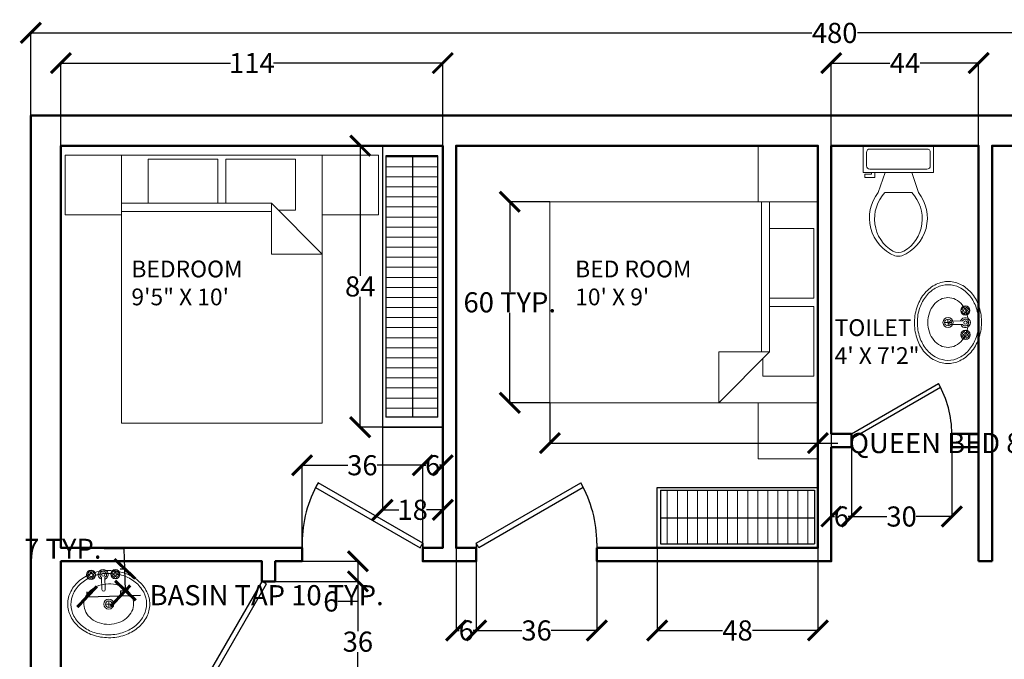
# Model space of a CAD drawing. Units: inches. Extents: x 9 to 573, y -373 to 44.
# Tile 3 of 5: x 35 to 329, y -146 to 44. Entities that reach past the tile are written whole.
import ezdxf

# ---------------------------------------------------------------- set-up
doc = ezdxf.new("R2010")
doc.units = ezdxf.units.IN
doc.header["$MEASUREMENT"] = 0
for name, color, linetype, lineweight in [('A-ANNO-DIMS', 2, 'Continuous', 18), ('A-AREA-IDEN', 7, 'Continuous', 25), ('A-DOOR', 4, 'Continuous', 25), ('A-FLOR-CASE', 8, 'Continuous', 25), ('A-FLOR-CASE-PATT', 252, 'Continuous', 13), ('A-FLOR-FIXT', 9, 'Continuous', 18), ('A-FURN', 8, 'Continuous', 18), ('A-WALL', 7, 'Continuous', 50)]:
    doc.layers.add(name, color=color, linetype=linetype, lineweight=lineweight)
doc.styles.get("Standard").update_dxf_attribs({"font": 'arial.ttf'})
doc.dimstyles.get("Standard").update_dxf_attribs({"dimtxt": 6, "dimasz": 6, "dimexe": 0.18, "dimexo": 0.0625, "dimgap": 0.09, "dimtad": 0, "dimtih": 1, "dimtoh": 1, "dimdec": 0, "dimzin": 0, "dimdsep": 46, "dimlunit": 4, "dimtxsty": 'Standard', "dimblk": 'ARCHTICK', "dimcen": 0.09, "dimadec": 0, "dimazin": 0, "dimtfac": 1, "dimtdec": 0, "dimtofl": 0, "dimtmove": 0, "dimatfit": 3, "dimldrblk": 'ARCHTICK', "dimfxl": 1, "dimtolj": 1, "dimtzin": 0, "dimarcsym": 0})

# ---------------------------------------------------------------- blocks, each defined once
blk = doc.blocks.new('*U5')
for p, q in [((0, 0), (0, -6)), ((-40, 0), (-40, -6))]:
    blk.add_line(p, q)
blk.add_lwpolyline([(0, 0), (-34.64, 20), (-35.52, 18.48), (-0.88, -1.52)], close=True)
blk.add_arc((0, 0), 40, 150, 180)
blk = doc.blocks.new('*U4')
for p, q in [((0, 0), (0, -6)), ((40, 0), (40, -6))]:
    blk.add_line(p, q)
blk.add_lwpolyline([(0, 0), (34.64, 20), (35.52, 18.48), (0.88, -1.52)], close=True)
blk.add_arc((0, 0), 40, 0, 30)
blk = doc.blocks.new('*U7')
for p, q in [((0, 0), (0, -6)), ((40, 0), (40, -6))]:
    blk.add_line(p, q)
blk.add_lwpolyline([(0, 0), (34.64, 20), (35.52, 18.48), (0.87, -1.52)], close=True)
blk.add_arc((0, 0), 40, 0, 30)
blk = doc.blocks.new('Bed - Queen')
for p, q in [((0, -80.00003), (0, 0)), ((0, 0), (59.99999, 0)), ((59.99999, 0), (59.99999, -80.00003)), ((7.99999, -1.2), (28.79998, -1.2)), ((7.99999, -14.4), (7.99999, -1.2)), ((28.79998, -1.2), (28.79998, -14.4)), ((31.19999, -1.2), (51.99999, -1.2)), ((31.19999, -14.4), (31.19999, -1.2)), ((51.99999, -1.2), (51.99999, -16.4)), ((0, -14.4), (44.8, -14.4)), ((59.99999, -29.6), (44.8, -14.4)), ((44.8, -14.4), (44.8, -29.6)), ((44.8, -16.8), (0, -16.8)), ((51.99999, -16.4), (46.79936, -16.4)), ((44.8, -29.6), (59.99999, -29.6)), ((59.99999, -80.00003), (0, -80.00003))]:
    blk.add_line(p, q)
blk = doc.blocks.new('Toilet - top')
for p, q in [((9.5, -6), (9.5, -2)), ((-10, -8.5), (-8, -8.5)), ((-10, -9.5), (-10, -8.5)), ((-8, -8.5), (-8, -8)), ((-7, -8), (-7, -9.5)), ((-4, -8), (-6, -14)), ((4, -8), (6, -14)), ((-7, -9.5), (-10, -9.5)), ((4, -14), (-4, -14))]:
    blk.add_line(p, q)
blk.add_lwpolyline([(10.5, -8), (10.5, 0), (-10.5, 0), (-10.5, -8)], close=True)
for points in [[(-9.5, -2), (-9.5, -6)], [(8.5, -1), (-8.5, -1)], [(-8.5, -7), (8.5, -7)]]:
    blk.add_lwpolyline(points)
for centre, radius, start, end in [((-8.62, -1.88), 0.884, 81.8699, 188.1301), ((8.62, -1.88), 0.884, 351.8699, 98.1301), ((-8.62, -6.12), 0.884, 171.8699, 278.1301), ((8.62, -6.12), 0.884, 261.8699, 8.1301), ((3.52, -21.58), 12.17, 141.4691, 247.9714), ((4.2, -21.82), 11.33, 136.3677, 238.9468), ((-3.52, -21.58), 12.17, 292.0284, 38.5307), ((-4.2, -21.82), 11.33, 301.053, 43.6321), ((0, -27.88), 4, 245.7318, 294.2682), ((0, -29), 4, 254.8605, 285.1395)]:
    blk.add_arc(centre, radius, start, end)
blk = doc.blocks.new('Sink - Oval top')
for p, q in [((-1, 0), (1, 0)), ((0, 1), (0, -1))]:
    blk.add_line(p, q)
for points in [[(-12.23, 0.39, 0.117634), (-11.46, -3.36, 0.104469), (-8.88, -6.8, 0.090016), (-5.08, -9.07, 0.08192), (-0.32, -10.02, 0.08192), (4.49, -9.38, 0.090016), (8.42, -7.36, 0.104469), (11.22, -4.09, 0.117634), (12.23, -0.39, 0.117634), (11.46, 3.36, 0.104469), (8.88, 6.8, 0.090016), (5.08, 9.07, 0.08192), (0.32, 10.02, 0.08192), (-4.49, 9.38, 0.090016), (-8.42, 7.36, 0.104469), (-11.22, 4.09, 0.117634)], [(-11.29, 0.16, 0.118622), (-10.52, -3.25, 0.104678), (-8.07, -6.36, 0.089562), (-4.54, -8.37, 0.081185), (-0.13, -9.15, 0.081185), (4.3, -8.49, 0.089562), (7.89, -6.58, 0.104678), (10.42, -3.55, 0.118622), (11.29, -0.16, 0.118622), (10.52, 3.25, 0.104678), (8.07, 6.36, 0.089562), (4.54, 8.37, 0.081185), (0.13, 9.15, 0.081185), (-4.3, 8.49, 0.089562), (-7.89, 6.58, 0.104678), (-10.42, 3.55, 0.118622)], [(-7.42, 0.08, 0.118283), (-6.91, -2.17, 0.104607), (-5.29, -4.21, 0.089718), (-2.97, -5.53, 0.081436), (-0.07, -6.04, 0.081436), (2.84, -5.59, 0.089718), (5.2, -4.33, 0.104607), (6.86, -2.32, 0.118283), (7.42, -0.08, 0.118283), (6.91, 2.17, 0.104607), (5.29, 4.21, 0.089718), (2.97, 5.53, 0.081436), (0.07, 6.04, 0.081436), (-2.84, 5.59, 0.089718), (-5.2, 4.33, 0.104607), (-6.86, 2.32, 0.118283)]]:
    blk.add_lwpolyline(points, format="xyb", close=True)
for radius in [1.5, 1]:
    blk.add_circle((0, 0), radius)
blk = doc.blocks.new('Faucet - Bathroom top')
for p, q in [((-4.107, 0.125), (-4.375, 0.125)), ((-3.75, 0.4788), (-3.75, 0.75)), ((-3.5, 0.482), (-3.5, 0.75)), ((-3.1461, 0.125), (-2.875, 0.125)), ((3.143, 0.125), (2.875, 0.125)), ((3.5, 0.4788), (3.5, 0.75)), ((3.75, 0.482), (3.75, 0.75)), ((4.1039, 0.125), (4.375, 0.125)), ((-4.1039, -0.125), (-4.375, -0.125)), ((-3.75, -0.4821), (-3.75, -0.75)), ((-3.5, -0.4789), (-3.5, -0.75)), ((-3.143, -0.125), (-2.875, -0.125)), ((-0.5, -0.8639), (-0.5, -4.5)), ((0.5, -4.5), (0.5, -0.8631)), ((3.1461, -0.125), (2.875, -0.125)), ((3.5, -0.4821), (3.5, -0.75)), ((3.75, -0.4789), (3.75, -0.75)), ((4.107, -0.125), (4.375, -0.125))]:
    blk.add_line(p, q)
for centre, radius in [((-3.625, 0), 1.375), ((-4.625, 0), 0.2795), ((-3.625, 0), 0.5), ((-3.625, 1), 0.2795), ((-2.625, 0), 0.2795), ((0, 0), 0.5), ((3.625, 0), 1.375), ((2.625, 0), 0.2795), ((3.625, 0), 0.5), ((3.625, 1), 0.2795), ((4.625, 0), 0.2795), ((-3.625, -1), 0.2795), ((3.625, -1), 0.2795)]:
    blk.add_circle(centre, radius)
for centre, radius, start, end in [((-3.625, 0), 1, 105.2407, 164.2093), ((-3.625, 0), 1, 16.44125, 74.07887), ((0, 0), 1.5, 289.6514, 250.3603), ((0, 0), 1, 300.3431, 239.7554), ((3.625, 0), 1, 106.12, 164.0884), ((3.625, 0), 1, 16.23422, 73.90469), ((-3.625, 0), 1, 196.2342, 253.9047), ((-3.625, 0), 1, 286.12, 344.0884), ((3.625, 0), 1, 196.4413, 254.0789), ((3.625, 0), 1, 285.2407, 344.2093), ((0, -4.5), 0.5, 180, 0)]:
    blk.add_arc(centre, radius, start, end)
blk = doc.blocks.new('*U25')
for p, q in [((0, 0), (0, 6)), ((40, 0), (40, 6))]:
    blk.add_line(p, q)
blk.add_lwpolyline([(0, 0), (34.64, -20), (35.52, -18.48), (0.87, 1.52)], close=True)
blk.add_arc((0, 0), 40, 330, 0)
blk = doc.blocks.new('BEDSIDE-TABLE')
blk.add_lwpolyline([(0, 17.82), (16.74, 17.82), (16.74, 0), (0, 0)], close=True)
blk = doc.blocks.new('_ArchTick')
at = {"color": 0, "linetype": 'ByBlock', "const_width": 0.15}
blk.add_lwpolyline([(-0.5, -0.5), (0.5, 0.5)], dxfattribs=at)
blk = doc.blocks.new('*D30')
at = {"layer": 'A-ANNO-DIMS', "color": 0, "lineweight": -2, "transparency": 16777216}
for p, q in [((193.52, -70), (193.52, -82.12)), ((273.52, -70), (273.52, -82.12)), ((193.52, -81.94), (273.52, -81.94)), ((273.52, -81.94), (279.52, -81.94))]:
    blk.add_line(p, q, dxfattribs=at)
at = {"layer": 'Defpoints', "color": 0, "transparency": 16777216}
for p in [(193.52, -69.94), (273.52, -69.94), (273.52, -81.94)]:
    blk.add_point(p, dxfattribs=at)
at = {"layer": 'A-ANNO-DIMS', "color": 0, "lineweight": -2, "transparency": 16777216, "xscale": 6, "yscale": 6, "zscale": 6, "rotation": 180}
blk.add_blockref('_ArchTick', (193.52, -81.94), dxfattribs=at)
at = {"layer": 'A-ANNO-DIMS', "color": 0, "lineweight": -2, "transparency": 16777216, "xscale": 6, "yscale": 6, "zscale": 6}
blk.add_blockref('_ArchTick', (273.52, -81.94), dxfattribs=at)
at = {"layer": 'A-ANNO-DIMS', "color": 0, "transparency": 16777216, "insert": (320.05, -81.94), "char_height": 6, "attachment_point": 5}
blk.add_mtext('\\A1;QUEEN BED 80 TYP.', dxfattribs=at)
blk = doc.blocks.new('*D31')
at = {"layer": 'A-ANNO-DIMS', "color": 0, "lineweight": -2, "transparency": 16777216}
for p, q in [((193.45, -9.94), (181.34, -9.94)), ((181.52, -9.94), (181.52, -36.78)), ((181.52, -69.94), (181.52, -43.09)), ((193.45, -69.94), (181.34, -69.94))]:
    blk.add_line(p, q, dxfattribs=at)
at = {"layer": 'Defpoints', "color": 0, "transparency": 16777216}
for p in [(193.52, -9.94), (181.52, -69.94), (193.52, -69.94)]:
    blk.add_point(p, dxfattribs=at)
at = {"layer": 'A-ANNO-DIMS', "color": 0, "lineweight": -2, "transparency": 16777216, "xscale": 6, "yscale": 6, "zscale": 6}
for p, rotation in [((181.52, -9.94), 90), ((181.52, -69.94), 270)]:
    blk.add_blockref('_ArchTick', p, dxfattribs=dict(at, rotation=rotation))
at = {"layer": 'A-ANNO-DIMS', "color": 0, "transparency": 16777216, "insert": (181.52, -39.94), "char_height": 6, "attachment_point": 5}
blk.add_mtext('\\A1;60 TYP.', dxfattribs=at)
blk = doc.blocks.new('*D40')
at = {"layer": 'A-ANNO-DIMS', "color": 0, "lineweight": -2, "transparency": 16777216}
for p, q in [((55.28, -126.35), (55.32, -127.97)), ((65.27, -126.07), (65.32, -127.68)), ((55.32, -127.79), (65.31, -127.5)), ((65.31, -127.5), (71.31, -127.33))]:
    blk.add_line(p, q, dxfattribs=at)
at = {"layer": 'Defpoints', "color": 0, "transparency": 16777216}
for p in [(55.28, -126.29), (65.27, -126.01), (65.31, -127.5)]:
    blk.add_point(p, dxfattribs=at)
at = {"layer": 'A-ANNO-DIMS', "color": 0, "lineweight": -2, "transparency": 16777216, "xscale": 6, "yscale": 6, "zscale": 6}
for p, rotation in [((55.32, -127.79), 181.633858055105), ((65.31, -127.5), 1.633858055105019)]:
    blk.add_blockref('_ArchTick', p, dxfattribs=dict(at, rotation=rotation))
at = {"layer": 'A-ANNO-DIMS', "color": 0, "transparency": 16777216, "insert": (108.93, -127.33), "char_height": 6, "attachment_point": 5}
blk.add_mtext('\\A1;BASIN TAP 10 TYP.', dxfattribs=at)
blk = doc.blocks.new('*D41')
at = {"layer": 'A-ANNO-DIMS', "color": 0, "lineweight": -2, "transparency": 16777216}
for p, q in [((66.41, -113.47), (60.41, -113.47)), ((66.59, -119.47), (66.41, -113.47)), ((65.15, -119.51), (66.77, -119.46)), ((66.77, -125.96), (66.59, -119.47)), ((65.33, -126), (66.95, -125.96))]:
    blk.add_line(p, q, dxfattribs=at)
at = {"layer": 'Defpoints', "color": 0, "transparency": 16777216}
for p in [(65.09, -119.51), (66.59, -119.47), (65.27, -126.01)]:
    blk.add_point(p, dxfattribs=at)
at = {"layer": 'A-ANNO-DIMS', "color": 0, "lineweight": -2, "transparency": 16777216, "xscale": 6, "yscale": 6, "zscale": 6}
for p, rotation in [((66.59, -119.47), 91.63385805510502), ((66.77, -125.96), 271.633858055105)]:
    blk.add_blockref('_ArchTick', p, dxfattribs=dict(at, rotation=rotation))
at = {"layer": 'A-ANNO-DIMS', "color": 0, "transparency": 16777216, "insert": (48.08, -113.47), "char_height": 6, "attachment_point": 5}
blk.add_mtext('\\A1;7 TYP.', dxfattribs=at)
blk = doc.blocks.new('*D58')
at = {"layer": 'A-ANNO-DIMS', "color": 0, "lineweight": -2, "transparency": 16777216}
for p, q in [((38.52, 15.87), (38.52, 40.63)), ((38.52, 40.45), (271.69, 40.45)), ((518.52, 40.45), (285.35, 40.45)), ((518.52, 15.87), (518.52, 40.63))]:
    blk.add_line(p, q, dxfattribs=at)
at = {"layer": 'Defpoints', "color": 0, "transparency": 16777216}
for p in [(518.52, 40.45), (38.52, 15.8), (518.52, 15.8)]:
    blk.add_point(p, dxfattribs=at)
at = {"layer": 'A-ANNO-DIMS', "color": 0, "lineweight": -2, "transparency": 16777216, "xscale": 6, "yscale": 6, "zscale": 6, "rotation": 180}
blk.add_blockref('_ArchTick', (38.52, 40.45), dxfattribs=at)
at = {"layer": 'A-ANNO-DIMS', "color": 0, "lineweight": -2, "transparency": 16777216, "xscale": 6, "yscale": 6, "zscale": 6}
blk.add_blockref('_ArchTick', (518.52, 40.45), dxfattribs=at)
at = {"layer": 'A-ANNO-DIMS', "color": 0, "transparency": 16777216, "insert": (278.52, 40.45), "char_height": 6, "attachment_point": 5}
blk.add_mtext('\\A1;480', dxfattribs=at)
blk = doc.blocks.new('*D68')
at = {"layer": 'A-ANNO-DIMS', "color": 0, "lineweight": -2, "transparency": 16777216}
for p, q in [((277.52, 6.87), (277.52, 31.63)), ((277.52, 31.45), (295.02, 31.45)), ((321.52, 31.45), (304.01, 31.45)), ((321.52, 6.87), (321.52, 31.63))]:
    blk.add_line(p, q, dxfattribs=at)
at = {"layer": 'Defpoints', "color": 0, "transparency": 16777216}
for p in [(321.52, 31.45), (277.52, 6.8), (321.52, 6.8)]:
    blk.add_point(p, dxfattribs=at)
at = {"layer": 'A-ANNO-DIMS', "color": 0, "lineweight": -2, "transparency": 16777216, "xscale": 6, "yscale": 6, "zscale": 6, "rotation": 180}
blk.add_blockref('_ArchTick', (277.52, 31.45), dxfattribs=at)
at = {"layer": 'A-ANNO-DIMS', "color": 0, "lineweight": -2, "transparency": 16777216, "xscale": 6, "yscale": 6, "zscale": 6}
blk.add_blockref('_ArchTick', (321.52, 31.45), dxfattribs=at)
at = {"layer": 'A-ANNO-DIMS', "color": 0, "transparency": 16777216, "insert": (299.52, 31.45), "char_height": 6, "attachment_point": 5}
blk.add_mtext('\\A1;44', dxfattribs=at)
blk = doc.blocks.new('*D69')
at = {"layer": 'A-ANNO-DIMS', "color": 0, "lineweight": -2, "transparency": 16777216}
for p, q in [((47.52, 6.87), (47.52, 31.63)), ((47.52, 31.45), (98.09, 31.45)), ((161.52, 31.45), (110.94, 31.45)), ((161.52, 6.87), (161.52, 31.63))]:
    blk.add_line(p, q, dxfattribs=at)
at = {"layer": 'Defpoints', "color": 0, "transparency": 16777216}
for p in [(161.52, 31.45), (47.52, 6.8), (161.52, 6.8)]:
    blk.add_point(p, dxfattribs=at)
at = {"layer": 'A-ANNO-DIMS', "color": 0, "lineweight": -2, "transparency": 16777216, "xscale": 6, "yscale": 6, "zscale": 6, "rotation": 180}
blk.add_blockref('_ArchTick', (47.52, 31.45), dxfattribs=at)
at = {"layer": 'A-ANNO-DIMS', "color": 0, "lineweight": -2, "transparency": 16777216, "xscale": 6, "yscale": 6, "zscale": 6}
blk.add_blockref('_ArchTick', (161.52, 31.45), dxfattribs=at)
at = {"layer": 'A-ANNO-DIMS', "color": 0, "transparency": 16777216, "insert": (104.52, 31.45), "char_height": 6, "attachment_point": 5}
blk.add_mtext('\\A1;114', dxfattribs=at)
blk = doc.blocks.new('*D70')
at = {"layer": 'A-ANNO-DIMS', "color": 0, "lineweight": -2, "transparency": 16777216}
for p, q in [((119.52, -113.13), (119.52, -88.37)), ((119.52, -88.55), (133.13, -88.55)), ((155.52, -88.55), (141.9, -88.55)), ((155.52, -113.13), (155.52, -88.37))]:
    blk.add_line(p, q, dxfattribs=at)
at = {"layer": 'Defpoints', "color": 0, "transparency": 16777216}
for p in [(155.52, -88.55), (119.52, -113.2), (155.52, -113.2)]:
    blk.add_point(p, dxfattribs=at)
at = {"layer": 'A-ANNO-DIMS', "color": 0, "lineweight": -2, "transparency": 16777216, "xscale": 6, "yscale": 6, "zscale": 6, "rotation": 180}
blk.add_blockref('_ArchTick', (119.52, -88.55), dxfattribs=at)
at = {"layer": 'A-ANNO-DIMS', "color": 0, "lineweight": -2, "transparency": 16777216, "xscale": 6, "yscale": 6, "zscale": 6}
blk.add_blockref('_ArchTick', (155.52, -88.55), dxfattribs=at)
at = {"layer": 'A-ANNO-DIMS', "color": 0, "transparency": 16777216, "insert": (137.52, -88.55), "char_height": 6, "attachment_point": 5}
blk.add_mtext('\\A1;36', dxfattribs=at)
blk = doc.blocks.new('*D71')
at = {"layer": 'A-ANNO-DIMS', "color": 0, "lineweight": -2, "transparency": 16777216}
for p, q in [((155.52, -113.13), (155.52, -88.37)), ((155.52, -88.55), (156.45, -88.55)), ((161.52, -88.55), (160.59, -88.55)), ((161.52, -113.13), (161.52, -88.37))]:
    blk.add_line(p, q, dxfattribs=at)
at = {"layer": 'Defpoints', "color": 0, "transparency": 16777216}
for p in [(161.52, -88.55), (155.52, -113.2), (161.52, -113.2)]:
    blk.add_point(p, dxfattribs=at)
at = {"layer": 'A-ANNO-DIMS', "color": 0, "lineweight": -2, "transparency": 16777216, "xscale": 6, "yscale": 6, "zscale": 6, "rotation": 180}
blk.add_blockref('_ArchTick', (155.52, -88.55), dxfattribs=at)
at = {"layer": 'A-ANNO-DIMS', "color": 0, "lineweight": -2, "transparency": 16777216, "xscale": 6, "yscale": 6, "zscale": 6}
blk.add_blockref('_ArchTick', (161.52, -88.55), dxfattribs=at)
at = {"layer": 'A-ANNO-DIMS', "color": 0, "transparency": 16777216, "insert": (158.52, -88.55), "char_height": 6, "attachment_point": 5}
blk.add_mtext('\\A1;6', dxfattribs=at)
blk = doc.blocks.new('*D72')
at = {"layer": 'A-ANNO-DIMS', "color": 0, "lineweight": -2, "transparency": 16777216}
for p, q in [((283.52, -79.26), (283.52, -104.03)), ((313.52, -79.26), (313.52, -104.03)), ((283.52, -103.85), (294.14, -103.85)), ((313.52, -103.85), (302.89, -103.85))]:
    blk.add_line(p, q, dxfattribs=at)
at = {"layer": 'Defpoints', "color": 0, "transparency": 16777216}
for p in [(283.52, -79.2), (313.52, -79.2), (283.52, -103.85)]:
    blk.add_point(p, dxfattribs=at)
at = {"layer": 'A-ANNO-DIMS', "color": 0, "lineweight": -2, "transparency": 16777216, "xscale": 6, "yscale": 6, "zscale": 6, "rotation": 180}
blk.add_blockref('_ArchTick', (283.52, -103.85), dxfattribs=at)
at = {"layer": 'A-ANNO-DIMS', "color": 0, "lineweight": -2, "transparency": 16777216, "xscale": 6, "yscale": 6, "zscale": 6}
blk.add_blockref('_ArchTick', (313.52, -103.85), dxfattribs=at)
at = {"layer": 'A-ANNO-DIMS', "color": 0, "transparency": 16777216, "insert": (298.52, -103.85), "char_height": 6, "attachment_point": 5}
blk.add_mtext('\\A1;30', dxfattribs=at)
blk = doc.blocks.new('*D73')
at = {"layer": 'A-ANNO-DIMS', "color": 0, "lineweight": -2, "transparency": 16777216}
for p, q in [((277.52, -79.26), (277.52, -104.03)), ((283.52, -79.26), (283.52, -104.03)), ((277.52, -103.85), (278.45, -103.85)), ((283.52, -103.85), (282.59, -103.85))]:
    blk.add_line(p, q, dxfattribs=at)
at = {"layer": 'Defpoints', "color": 0, "transparency": 16777216}
for p in [(277.52, -79.2), (283.52, -79.2), (277.52, -103.85)]:
    blk.add_point(p, dxfattribs=at)
at = {"layer": 'A-ANNO-DIMS', "color": 0, "lineweight": -2, "transparency": 16777216, "xscale": 6, "yscale": 6, "zscale": 6}
for p, rotation in [((277.52, -103.85), 179.9999999999999), ((283.52, -103.85), 359.9999999999999)]:
    blk.add_blockref('_ArchTick', p, dxfattribs=dict(at, rotation=rotation))
at = {"layer": 'A-ANNO-DIMS', "color": 0, "transparency": 16777216, "insert": (280.52, -103.85), "char_height": 6, "attachment_point": 5}
blk.add_mtext('\\A1;6', dxfattribs=at)
blk = doc.blocks.new('*D80')
at = {"layer": 'A-ANNO-DIMS', "color": 0, "lineweight": -2, "transparency": 16777216}
for p, q in [((111.58, -123.2), (136.35, -123.2)), ((136.17, -123.2), (136.17, -138.04)), ((136.17, -159.2), (136.17, -144.35)), ((111.58, -159.2), (136.35, -159.2))]:
    blk.add_line(p, q, dxfattribs=at)
at = {"layer": 'Defpoints', "color": 0, "transparency": 16777216}
for p in [(111.52, -123.2), (111.52, -159.2), (136.17, -159.2)]:
    blk.add_point(p, dxfattribs=at)
at = {"layer": 'A-ANNO-DIMS', "color": 0, "lineweight": -2, "transparency": 16777216, "xscale": 6, "yscale": 6, "zscale": 6}
for p, rotation in [((136.17, -123.2), 90), ((136.17, -159.2), 270)]:
    blk.add_blockref('_ArchTick', p, dxfattribs=dict(at, rotation=rotation))
at = {"layer": 'A-ANNO-DIMS', "color": 0, "transparency": 16777216, "insert": (136.17, -141.2), "char_height": 6, "attachment_point": 5}
blk.add_mtext('\\A1;36', dxfattribs=at)
blk = doc.blocks.new('*D81')
at = {"layer": 'A-ANNO-DIMS', "color": 0, "lineweight": -2, "transparency": 16777216}
for p, q in [((111.58, -117.2), (136.35, -117.2)), ((136.17, -117.2), (136.17, -123.2)), ((111.58, -123.2), (136.35, -123.2)), ((136.17, -123.2), (136.17, -129.2)), ((136.17, -129.2), (130.17, -129.2))]:
    blk.add_line(p, q, dxfattribs=at)
at = {"layer": 'Defpoints', "color": 0, "transparency": 16777216}
for p in [(111.52, -117.2), (111.52, -123.2), (136.17, -123.2)]:
    blk.add_point(p, dxfattribs=at)
at = {"layer": 'A-ANNO-DIMS', "color": 0, "lineweight": -2, "transparency": 16777216, "xscale": 6, "yscale": 6, "zscale": 6}
for p, rotation in [((136.17, -117.2), 90), ((136.17, -123.2), 270)]:
    blk.add_blockref('_ArchTick', p, dxfattribs=dict(at, rotation=rotation))
at = {"layer": 'A-ANNO-DIMS', "color": 0, "transparency": 16777216, "insert": (128.1, -129.2), "char_height": 6, "attachment_point": 5}
blk.add_mtext('\\A1;6', dxfattribs=at)
blk = doc.blocks.new('*D82')
at = {"layer": 'A-ANNO-DIMS', "color": 0, "lineweight": -2, "transparency": 16777216}
for p, q in [((165.52, -113.26), (165.52, -138.03)), ((171.52, -113.26), (171.52, -138.03)), ((165.52, -137.85), (166.45, -137.85)), ((171.52, -137.85), (170.59, -137.85))]:
    blk.add_line(p, q, dxfattribs=at)
at = {"layer": 'Defpoints', "color": 0, "transparency": 16777216}
for p in [(165.52, -113.2), (171.52, -113.2), (165.52, -137.85)]:
    blk.add_point(p, dxfattribs=at)
at = {"layer": 'A-ANNO-DIMS', "color": 0, "lineweight": -2, "transparency": 16777216, "xscale": 6, "yscale": 6, "zscale": 6, "rotation": 180}
blk.add_blockref('_ArchTick', (165.52, -137.85), dxfattribs=at)
at = {"layer": 'A-ANNO-DIMS', "color": 0, "lineweight": -2, "transparency": 16777216, "xscale": 6, "yscale": 6, "zscale": 6}
blk.add_blockref('_ArchTick', (171.52, -137.85), dxfattribs=at)
at = {"layer": 'A-ANNO-DIMS', "color": 0, "transparency": 16777216, "insert": (168.52, -137.85), "char_height": 6, "attachment_point": 5}
blk.add_mtext('\\A1;6', dxfattribs=at)
blk = doc.blocks.new('*D83')
at = {"layer": 'A-ANNO-DIMS', "color": 0, "lineweight": -2, "transparency": 16777216}
for p, q in [((171.52, -113.26), (171.52, -138.03)), ((207.52, -113.26), (207.52, -138.03)), ((171.52, -137.85), (185.13, -137.85)), ((207.52, -137.85), (193.9, -137.85))]:
    blk.add_line(p, q, dxfattribs=at)
at = {"layer": 'Defpoints', "color": 0, "transparency": 16777216}
for p in [(171.52, -113.2), (207.52, -113.2), (171.52, -137.85)]:
    blk.add_point(p, dxfattribs=at)
at = {"layer": 'A-ANNO-DIMS', "color": 0, "lineweight": -2, "transparency": 16777216, "xscale": 6, "yscale": 6, "zscale": 6, "rotation": 180}
blk.add_blockref('_ArchTick', (171.52, -137.85), dxfattribs=at)
at = {"layer": 'A-ANNO-DIMS', "color": 0, "lineweight": -2, "transparency": 16777216, "xscale": 6, "yscale": 6, "zscale": 6}
blk.add_blockref('_ArchTick', (207.52, -137.85), dxfattribs=at)
at = {"layer": 'A-ANNO-DIMS', "color": 0, "transparency": 16777216, "insert": (189.52, -137.85), "char_height": 6, "attachment_point": 5}
blk.add_mtext('\\A1;36', dxfattribs=at)
blk = doc.blocks.new('*D88')
at = {"layer": 'A-ANNO-DIMS', "color": 0, "lineweight": -2, "transparency": 16777216}
for p, q in [((161.45, 6.8), (136.69, 6.8)), ((136.87, 6.8), (136.87, -32.04)), ((136.87, -77.2), (136.87, -38.35)), ((161.45, -77.2), (136.69, -77.2))]:
    blk.add_line(p, q, dxfattribs=at)
at = {"layer": 'Defpoints', "color": 0, "transparency": 16777216}
for p in [(136.87, 6.8), (161.52, 6.8), (161.52, -77.2)]:
    blk.add_point(p, dxfattribs=at)
at = {"layer": 'A-ANNO-DIMS', "color": 0, "lineweight": -2, "transparency": 16777216, "xscale": 6, "yscale": 6, "zscale": 6}
for p, rotation in [((136.87, 6.8), 90), ((136.87, -77.2), 270)]:
    blk.add_blockref('_ArchTick', p, dxfattribs=dict(at, rotation=rotation))
at = {"layer": 'A-ANNO-DIMS', "color": 0, "transparency": 16777216, "insert": (136.87, -35.2), "char_height": 6, "attachment_point": 5}
blk.add_mtext('\\A1;84', dxfattribs=at)
blk = doc.blocks.new('*D89')
at = {"layer": 'A-ANNO-DIMS', "color": 0, "lineweight": -2, "transparency": 16777216}
for p, q in [((143.52, -77.26), (143.52, -102.03)), ((161.52, -77.26), (161.52, -102.03)), ((143.52, -101.85), (148.41, -101.85)), ((161.52, -101.85), (156.63, -101.85))]:
    blk.add_line(p, q, dxfattribs=at)
at = {"layer": 'Defpoints', "color": 0, "transparency": 16777216}
for p in [(143.52, -77.2), (161.52, -77.2), (143.52, -101.85)]:
    blk.add_point(p, dxfattribs=at)
at = {"layer": 'A-ANNO-DIMS', "color": 0, "lineweight": -2, "transparency": 16777216, "xscale": 6, "yscale": 6, "zscale": 6, "rotation": 180}
blk.add_blockref('_ArchTick', (143.52, -101.85), dxfattribs=at)
at = {"layer": 'A-ANNO-DIMS', "color": 0, "lineweight": -2, "transparency": 16777216, "xscale": 6, "yscale": 6, "zscale": 6}
blk.add_blockref('_ArchTick', (161.52, -101.85), dxfattribs=at)
at = {"layer": 'A-ANNO-DIMS', "color": 0, "transparency": 16777216, "insert": (152.52, -101.85), "char_height": 6, "attachment_point": 5}
blk.add_mtext('\\A1;18', dxfattribs=at)
blk = doc.blocks.new('*D90')
at = {"layer": 'A-ANNO-DIMS', "color": 0, "lineweight": -2, "transparency": 16777216}
for p, q in [((225.52, -113.26), (225.52, -138.03)), ((273.52, -113.26), (273.52, -138.03)), ((225.52, -137.85), (245, -137.85)), ((273.52, -137.85), (254.03, -137.85))]:
    blk.add_line(p, q, dxfattribs=at)
at = {"layer": 'Defpoints', "color": 0, "transparency": 16777216}
for p in [(225.52, -113.2), (273.52, -113.2), (225.52, -137.85)]:
    blk.add_point(p, dxfattribs=at)
at = {"layer": 'A-ANNO-DIMS', "color": 0, "lineweight": -2, "transparency": 16777216, "xscale": 6, "yscale": 6, "zscale": 6, "rotation": 180}
blk.add_blockref('_ArchTick', (225.52, -137.85), dxfattribs=at)
at = {"layer": 'A-ANNO-DIMS', "color": 0, "lineweight": -2, "transparency": 16777216, "xscale": 6, "yscale": 6, "zscale": 6}
blk.add_blockref('_ArchTick', (273.52, -137.85), dxfattribs=at)
at = {"layer": 'A-ANNO-DIMS', "color": 0, "transparency": 16777216, "insert": (249.52, -137.85), "char_height": 6, "attachment_point": 5}
blk.add_mtext('\\A1;48', dxfattribs=at)

msp = doc.modelspace()

# ---------------------------------------------------------------- hatches: boundary and pattern name
at = {"layer": 'A-FLOR-CASE-PATT'}
h = msp.add_hatch(dxfattribs=at)
h.set_pattern_fill('ANSI31', color=256, scale=24, angle=-45, style=0)
h.set_pattern_definition([(0, (-716.4455, -458.4915), (0, 3), [])])
h.paths.add_polyline_path([(144.5545, -74.1966), (160.0545, -74.1966), (160.0545, 3.8034), (144.5545, 3.8034)])
h = msp.add_hatch(dxfattribs=at)
h.set_pattern_fill('ANSI31', color=256, scale=24, angle=45, style=0)
h.set_pattern_definition([(90, (-716.4455, -458.4915), (-3, 0), [])])
h.paths.add_polyline_path([(226.5545, -111.9915), (272.5545, -111.9915), (272.5545, -95.9915), (226.5545, -95.9915)])

# ---------------------------------------------------------------- linework, layer by layer
at = {"layer": 'A-FLOR-CASE'}
for p, q in [((161.5169, 6.8034), (143.5169, 6.8034)), ((143.5169, 6.8034), (143.5169, -77.1966)), ((161.5169, -77.1966), (161.5169, 6.8034)), ((160.0545, 3.8034), (144.5545, 3.8034)), ((144.5545, 3.8034), (144.5545, -74.1966)), ((152.5169, 3.8034), (152.5169, -74.1966)), ((160.0545, -74.1966), (160.0545, 3.8034)), ((160.0545, -74.1966), (144.5545, -74.1966)), ((143.5169, -77.1966), (161.5169, -77.1966)), ((225.5169, -113.1966), (225.5169, -95.1966)), ((225.5169, -95.1966), (273.5169, -95.1966)), ((226.5545, -95.9915), (272.5545, -95.9915)), ((226.5545, -95.9915), (226.5545, -111.9915)), ((272.5545, -95.9915), (272.5545, -111.9915)), ((273.5169, -95.1966), (273.5169, -113.1966)), ((226.5545, -104.1966), (272.5545, -104.1966)), ((273.5169, -113.1966), (225.5169, -113.1966)), ((226.5545, -111.9915), (272.5545, -111.9915))]:
    msp.add_line(p, q, dxfattribs=at)
at = {"layer": 'A-WALL'}
for p, q in [((283.5169, -79.1966), (283.5169, -83.1966)), ((313.5169, -79.1966), (313.5169, -83.1966)), ((313.5169, -79.1966), (321.5169, -79.1966)), ((313.5169, -83.1966), (321.5169, -83.1966)), ((325.5169, -113.1966), (325.5169, -117.1966))]:
    msp.add_line(p, q, dxfattribs=at)
for points in [[(329.5169, -215.1966), (329.5169, -335.1966), (509.5169, -335.1966), (518.5169, -335.1966), (518.5169, -344.1966), (38.5169, -344.1966), (38.5169, 15.8034), (518.5169, 15.8034), (518.5169, -117.1966), (450.7536, -117.1966), (450.7536, -140.1966), (446.7536, -140.1966), (446.7536, -117.1966), (431.5169, -117.1966), (431.5169, -113.1966), (509.5169, -113.1966), (509.5169, 6.8034), (389.5169, 6.8034), (389.5169, -113.1966), (395.5169, -113.1966), (395.5169, -117.1966), (385.5169, -117.1966), (385.5169, 6.8034), (325.5169, 6.8034)], [(283.5169, -83.1966), (277.5169, -83.1966), (277.5169, -117.1966), (207.5169, -117.1966), (207.5169, -113.1966), (273.5169, -113.1966), (273.5169, 6.8034), (165.5169, 6.8034), (165.5169, -113.1966), (171.5169, -113.1966), (171.5169, -117.1966), (155.5169, -117.1966), (155.5169, -113.1966), (161.5169, -113.1966), (161.5169, 6.8034), (47.5169, 6.8034), (47.5169, -113.1966), (119.5169, -113.1966), (119.5169, -117.1966), (111.5169, -117.1966), (111.5169, -123.1966), (107.5169, -123.1966), (107.5169, -117.1966), (47.5169, -117.1966), (47.5169, -211.1966)], [(321.5169, -117.1966), (321.5169, 6.8034), (277.5169, 6.8034), (277.5169, -79.1966), (283.5169, -79.1966)], [(325.5169, -117.1966), (321.5169, -117.1966)]]:
    msp.add_lwpolyline(points, dxfattribs=at)
msp.add_lwpolyline([(325.5169, -113.1966), (325.5169, 6.8034)], close=True, dxfattribs=at)

# ---------------------------------------------------------------- block references
at = {"layer": 'A-DOOR'}
for name, p, xscale, yscale, zscale in [('*U7', (283.5169, -79.1966), 0.75, 0.75, 0.75), ('*U5', (155.5169, -111.7966), 0.9, 0.9, 0.9), ('*U4', (171.5169, -111.7966), 0.9, 0.9, 0.9)]:
    msp.add_blockref(name, p, dxfattribs=dict(at, xscale=xscale, yscale=yscale, zscale=zscale))
at = {"layer": 'A-DOOR', "xscale": 0.9, "yscale": 0.9, "zscale": 0.9, "rotation": 270}
msp.add_blockref('*U25', (107.5169, -123.1966), dxfattribs=at)
at = {"layer": 'A-FLOR-FIXT'}
msp.add_blockref('Toilet - top', (297.5545, 6.8034), dxfattribs=at)
for name, p, rotation in [('Sink - Oval top', (312.3645, -45.9644), 270.6375101586001), ('Faucet - Bathroom top', (317.5627, -45.9994), 270.6375101586001), ('Sink - Oval top', (61.7933, -129.9889), 1.633858055105068), ('Faucet - Bathroom top', (60.1311, -121.15), 1.633858055105068)]:
    msp.add_blockref(name, p, dxfattribs=dict(at, rotation=rotation))
at = {"layer": 'A-FURN', "rotation": 270}
for name, p in [('BEDSIDE-TABLE', (255.6923, 6.8038)), ('Bed - Queen', (273.5169, -9.9382)), ('BEDSIDE-TABLE', (255.6923, -69.9377))]:
    msp.add_blockref(name, p, dxfattribs=at)
at = {"layer": 'A-FURN'}
for name, p in [('BEDSIDE-TABLE', (48.8124, -13.816)), ('Bed - Queen', (65.5545, 4.0085)), ('BEDSIDE-TABLE', (125.554, -13.816))]:
    msp.add_blockref(name, p, dxfattribs=at)

# ---------------------------------------------------------------- texts
at = {"layer": 'A-AREA-IDEN', "char_height": 5, "attachment_point": 1}
for s, width, insert in [('BEDROOM \\P9\'5" X 10\'', 56.999995, (68.5545, -27.4915)), ("BED ROOM \\P10' X 9'", 55.662405, (201.0545, -27.4915)), ('TOILET\\P4\' X 7\'2"', 44, (278.5169, -44.9915))]:
    msp.add_mtext_dynamic_manual_height_columns(s, width=width, gutter_width=1, heights=[0], dxfattribs=dict(at, insert=insert))

# ---------------------------------------------------------------- dimensions: what is measured, and where the dimension line sits
at = {"layer": 'A-ANNO-DIMS'}
for base, p1, p2, picture, middle in [((518.5169, 40.4534), (38.5169, 15.8034), (518.5169, 15.8034), '*D58', (278.5169, 40.4534)), ((161.5169, 31.4534), (47.5169, 6.8034), (161.5169, 6.8034), '*D69', (104.5169, 31.4534)), ((321.5169, 31.4534), (277.5169, 6.8034), (321.5169, 6.8034), '*D68', (299.5169, 31.4534)), ((155.5169, -88.5466), (119.5169, -113.1966), (155.5169, -113.1966), '*D70', (137.5169, -88.5466)), ((161.5169, -88.5466), (155.5169, -113.1966), (161.5169, -113.1966), '*D71', (158.5169, -88.5466))]:
    dim = msp.add_linear_dim(base=base, p1=p1, p2=p2, dimstyle='Standard', override={"dimdec": 0, "dimlfac": 1, "dimrnd": 0, "dimzin": 0, "dimdsep": 46, "dimlunit": 2}, dxfattribs=at)
    dim.commit()
    dim.dimension.update_dxf_attribs({"geometry": picture, "text_midpoint": middle})
for base, p1, p2, angle, picture, middle in [((136.8669, 6.8034), (161.5169, -77.1966), (161.5169, 6.8034), 90, '*D88', (136.8669, -35.1966)), ((143.5169, -101.8466), (161.5169, -77.1966), (143.5169, -77.1966), 180, '*D89', (152.5169, -101.8466)), ((277.5169, -103.8466), (283.5169, -79.1966), (277.5169, -79.1966), 180, '*D73', (280.5169, -103.8466)), ((283.5169, -103.8466), (313.5169, -79.1966), (283.5169, -79.1966), 180, '*D72', (298.5169, -103.8466)), ((136.1669, -123.1966), (111.5169, -117.1966), (111.5169, -123.1966), 270, '*D81', (128.096, -129.1966)), ((165.5169, -137.8466), (171.5169, -113.1966), (165.5169, -113.1966), 180, '*D82', (168.5169, -137.8466)), ((171.5169, -137.8466), (207.5169, -113.1966), (171.5169, -113.1966), 180, '*D83', (189.5169, -137.8466)), ((225.5169, -137.8466), (273.5169, -113.1966), (225.5169, -113.1966), 180, '*D90', (249.5169, -137.8466)), ((136.1669, -159.1966), (111.5169, -123.1966), (111.5169, -159.1966), 270, '*D80', (136.1669, -141.1966))]:
    dim = msp.add_linear_dim(base=base, p1=p1, p2=p2, angle=angle, dimstyle='Standard', override={"dimdec": 0, "dimlfac": 1, "dimrnd": 0, "dimzin": 0, "dimdsep": 46, "dimlunit": 2}, dxfattribs=at)
    dim.commit()
    dim.dimension.update_dxf_attribs({"geometry": picture, "text_midpoint": middle})
for base, p1, p2, angle, text, picture, middle in [((181.5168, -69.9382), (193.5168, -9.9382), (193.5168, -69.9382), 270, '<> TYP.', '*D31', (181.5168, -39.9382)), ((66.5857, -119.4652), (65.2716, -126.0054), (65.0863, -119.508), 91.633858, '<> TYP.', '*D41', (48.077, -113.4676)), ((65.3144, -127.5048), (55.2757, -126.2905), (65.2716, -126.0054), 1.633858, 'BASIN TAP <> TYP.', '*D40', (108.9285, -127.3337))]:
    dim = msp.add_linear_dim(base=base, p1=p1, p2=p2, angle=angle, text=text, dimstyle='Standard', override={"dimdec": 0, "dimlfac": 1, "dimrnd": 0, "dimzin": 0, "dimdsep": 46, "dimlunit": 2}, dxfattribs=at)
    dim.commit()
    dim.dimension.update_dxf_attribs({"geometry": picture, "text_midpoint": middle})
dim = msp.add_linear_dim(base=(273.5169, -81.9382), p1=(193.5168, -69.9382), p2=(273.5169, -69.9382), text='QUEEN BED <> TYP.', dimstyle='Standard', override={"dimdec": 0, "dimlfac": 1, "dimrnd": 0, "dimzin": 0, "dimdsep": 46, "dimlunit": 2}, dxfattribs=at)
dim.commit()
dim.dimension.update_dxf_attribs({"geometry": '*D30', "text_midpoint": (320.0537, -81.9382)})

doc.saveas('drawing.dxf')
